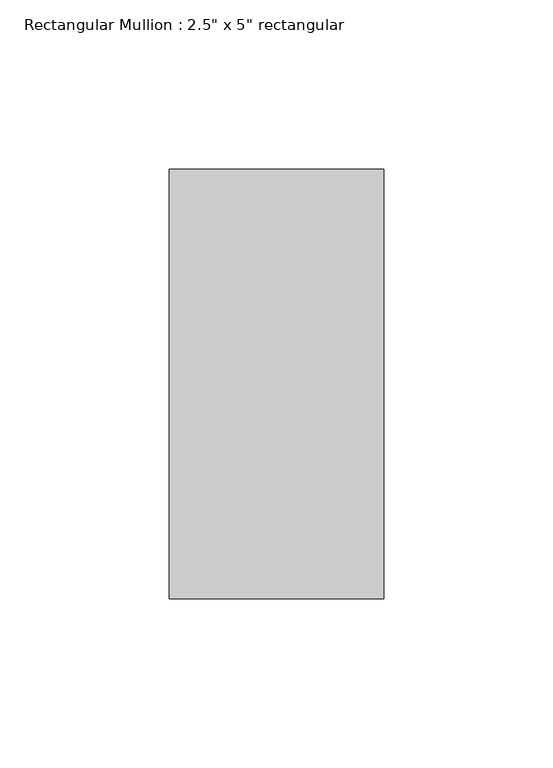
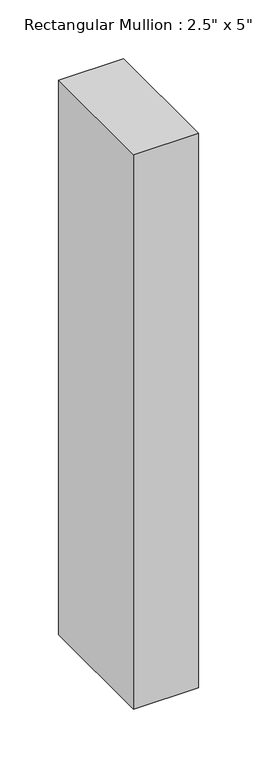
"""IFC4 building model written with IfcOpenShell, lengths in millimetres: member geometry."""

from ifc_helpers import new_model, si_unit, frame, origin, place, context, project, spatial, polyline, outline, extrude, source, transform, mapped, element, save


def member_8c893cff(model_context):
    return source(origin(), model_context, "Body", "SweptSolid", [
        extrude(outline(polyline([(0.0, 63.5), (0.0, -63.5), (-63.5, -63.5), (-63.5, 63.5), (0.0, 63.5)])), frame((0.0, 0.0, -574.266556), z_axis=(0.0, 0.0, 1.0), x_axis=(1.0, 0.0, 0.0)), (0.0, 0.0, 1.0), 574.266556),
    ])


if __name__ == "__main__":
    model = new_model("IFC4")
    model_context = context("Model", 3, world=origin())
    ifc_project = project(units=[si_unit("LENGTHUNIT", "METRE", prefix="MILLI")], contexts=[model_context])
    site = spatial("IfcSite", under=ifc_project)
    building = spatial("IfcBuilding", under=site)
    placement = place(None, origin())
    member_shape = member_8c893cff(model_context)
    element("IfcMember", 1, ObjectType="Rectangular Mullion : 2.5\" x 5\" rectangular", at=placement, inside=building, context=model_context, shape_type="MappedRepresentation", body=[
        mapped(member_shape, transform((0.0, 0.0, 0.0), x_axis=(1.0, 0.0, 0.0), y_axis=(0.0, 1.0, 0.0), z_axis=(0.0, 0.0, 1.0))),
    ])
    save(model, "model.ifc")

# Revit data of these elements
# Type "Rectangular Mullion : 2.5\" x 5\" rectangular"
#   built-in parameter 1007304 = 0.416667 (stored number, unit not read)
#   built-in parameter 1007301 = 0.104167 (stored number, unit not read)
#   built-in parameter 1007300 = 0.104167 (stored number, unit not read)
# Element 1 (IfcMember, "Rectangular Mullion : 2.5\" x 5\" rectangular")
#   Materials on its faces: "Aluminum"
# Materials
#   "Aluminum": class "Metal", colour RGB 247 247 247, transparency 0, Description = "Aluminum 6061", Cost = 0
